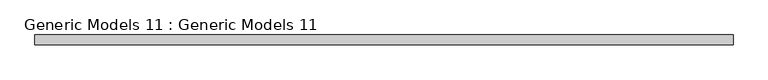
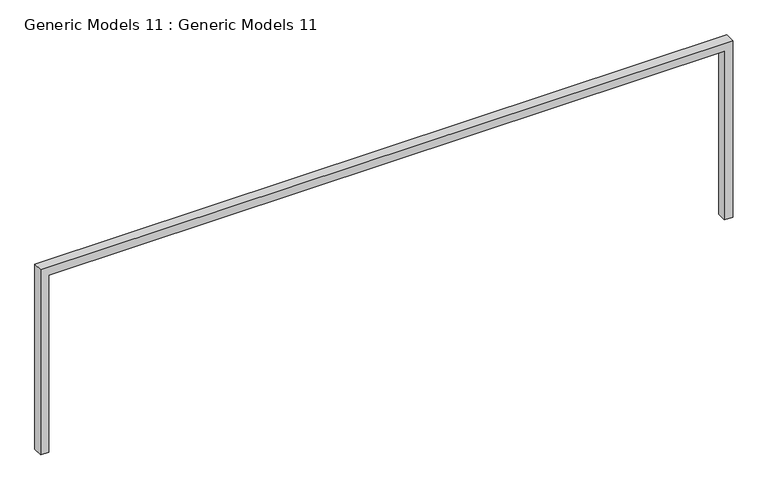
"""IFC4 building model written with IfcOpenShell, lengths in millimetres: proxy geometry, Generic Models 11 : Generic Models 11."""

from ifc_helpers import new_model, si_unit, frame, origin, place, context, project, spatial, polyline, outline, extrude, source, transform, mapped, element, save


def generic_models_11_generic_models_11_747a53b2(model_context):
    return source(origin(), model_context, "Body", "SweptSolid", [
        extrude(outline(polyline([(304.8, 1594.5748148), (304.8, 1734.2748148), (3421.0529412, 1734.2748148), (3421.0529412, -9832.2310677), (152.4, -9832.2310677), (152.4, -9692.5310677), (3281.3529412, -9692.5310677), (3281.3529412, 1594.5748148), (304.8, 1594.5748148)])), frame((0.0, -7442.2729199, 0.0), z_axis=(0.0, 1.0, 0.0), x_axis=(0.0, 0.0, 1.0)), (0.0, 0.0, 1.0), 165.1),
    ])


if __name__ == "__main__":
    model = new_model("IFC4")
    model_context = context("Model", 3, world=origin())
    ifc_project = project(units=[si_unit("LENGTHUNIT", "METRE", prefix="MILLI")], contexts=[model_context])
    site = spatial("IfcSite", under=ifc_project)
    building = spatial("IfcBuilding", under=site)
    placement = place(None, origin())
    generic_models_11_generic_models_11_shape = generic_models_11_generic_models_11_747a53b2(model_context)
    element("IfcBuildingElementProxy", 1, Name="Generic Models 11 : Generic Models 11", ObjectType="Generic Models 11 : Generic Models 11", at=placement, inside=building, context=model_context, shape_type="MappedRepresentation", body=[
        mapped(generic_models_11_generic_models_11_shape, transform((0.0, 0.0, 0.0), x_axis=(1.0, 0.0, 0.0), y_axis=(0.0, 1.0, 0.0), z_axis=(0.0, 0.0, 1.0))),
    ])
    save(model, "model.ifc")
